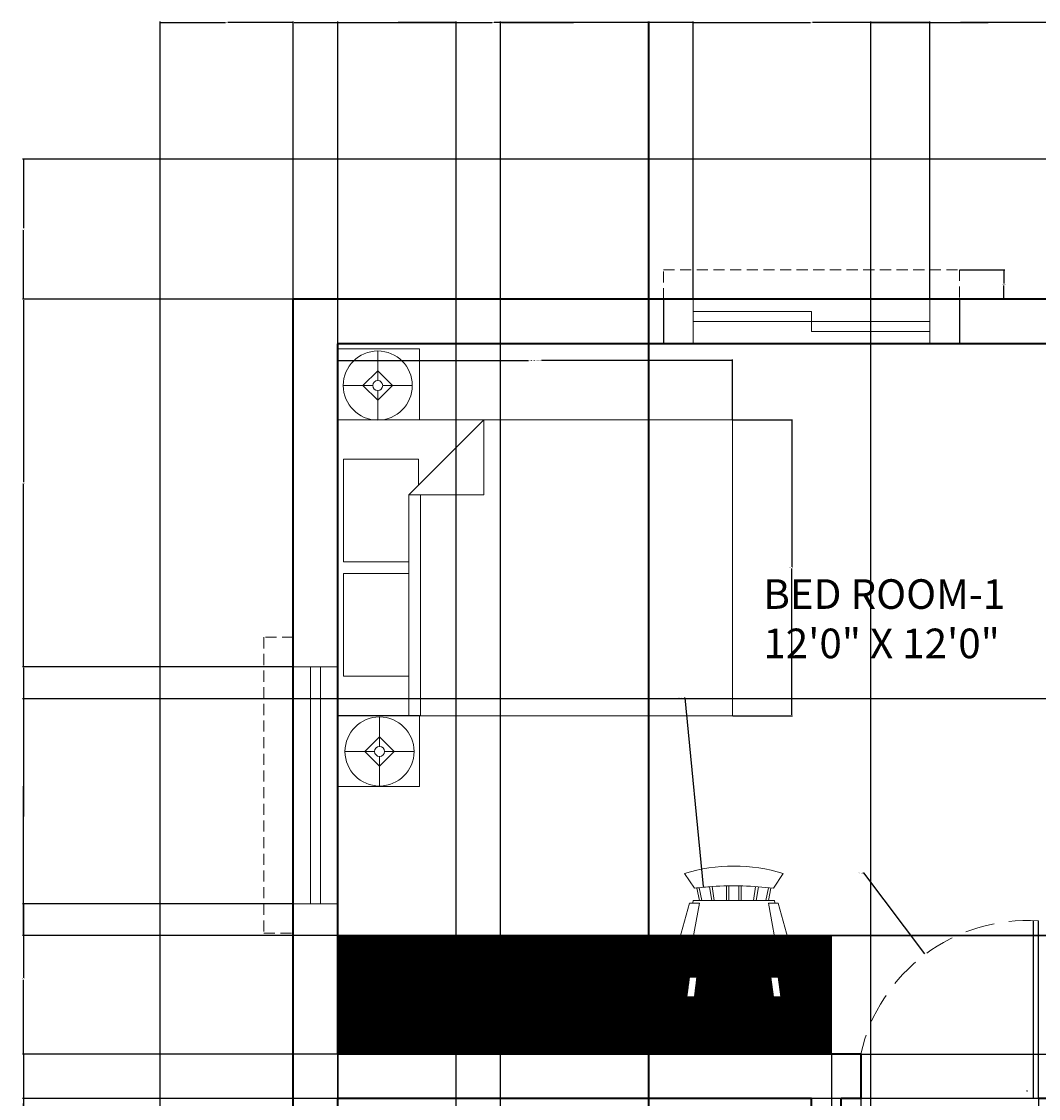
# Model space of a CAD drawing. Units: inches. Extents: x 6662 to 7211, y 5077 to 5683.
# Tile 7 of 9: x 6662 to 6868, y 5465 to 5683. Entities that reach past the tile are written whole.
import ezdxf

# ---------------------------------------------------------------- set-up
doc = ezdxf.new("R2010")
doc.units = ezdxf.units.IN
doc.header["$LTSCALE"] = 3
doc.header["$MEASUREMENT"] = 0
doc.linetypes.add('HIDDEN', pattern=[0.375, 0.25, -0.125])
for name, color, linetype, lineweight in [('A-ANNO-DIMS', 2, 'Continuous', 18), ('A-AREA-IDEN', 7, 'Continuous', 18), ('A-DOOR', 4, 'Continuous', 25), ('A-DOOR-HIDN', 4, 'HIDDEN', 13), ('A-FLOR-CASE', 8, 'Continuous', 20), ('A-FLOR-CASE-PATT', 241, 'Continuous', 13), ('A-FURN', 8, 'Continuous', 18), ('A-GLAZ', 4, 'Continuous', 18), ('A-GLAZ-OVHD', 4, 'HIDDEN', 13), ('A-WALL', 7, 'Continuous', 35)]:
    doc.layers.add(name, color=color, linetype=linetype, lineweight=lineweight)
doc.styles.get("Standard").update_dxf_attribs({"font": 'arial.ttf'})
doc.dimstyles.get("Standard").update_dxf_attribs({"dimtxt": 0.18, "dimasz": 0.18, "dimexe": 0.18, "dimexo": 0.0625, "dimgap": 0.09, "dimtad": 0, "dimtih": 1, "dimtoh": 1, "dimdec": 4, "dimzin": 0, "dimdsep": 46, "dimtxsty": 'Standard', "dimcen": 0.09, "dimadec": 0, "dimazin": 0, "dimtfac": 1, "dimtdec": 4, "dimtofl": 0, "dimtmove": 0, "dimatfit": 3, "dimfxl": 1, "dimtolj": 1, "dimtzin": 0, "dimarcsym": 0})

# ---------------------------------------------------------------- blocks, each defined once
blk = doc.blocks.new('Chair - Rocking')
for p, q in [((-8, -4.5), (-10, -1.5)), ((8, -4.5), (10, -1.5)), ((-4.5, -7), (-4.96674, -4.19951)), ((-4, -7), (-4.40532, -4.16272)), ((-1.5, -4.05012), (-1.5, -7)), ((-1, -7), (-1, -4.05012)), ((1, -7), (1, -4.04655)), ((1.5, -4.05012), (1.5, -7)), ((4, -7), (4.40187, -4.18694)), ((4.5, -7), (4.96761, -4.19437)), ((-7.5, -4.5), (-7, -7)), ((-6.5, -7), (-7.02225, -4.43)), ((6.5, -7), (7, -4.4057)), ((7.5, -4.5), (7, -7)), ((-9, -7.5), (-12, -18.49999)), ((-7, -7.5), (-9, -7.5)), ((-9, -18.49999), (-7, -7.5)), ((-8.23428, -6.99939), (-8.3093, -7.47958)), ((-8.23041, -7), (8.23915, -7)), ((7, -7.5), (9, -7.5)), ((9, -18.49999), (7, -7.5)), ((8.31071, -7.48854), (8.23449, -7.00073)), ((9, -7.5), (12, -18.49999)), ((-10.36644, -20.64523), (-10.5, -21.49999)), ((10.5, -21.49999), (10.3575, -20.58798)), ((-9, -22.49999), (-9.5, -26.49999)), ((0, -22.49999), (-9.5, -22.49999)), ((-8, -26.49999), (-7.5, -22.49999)), ((0, -22.49999), (9.5, -22.49999)), ((8, -26.49999), (7.5, -22.49999)), ((9, -22.49999), (9.5, -26.49999)), ((-9.5, -26.49999), (-8, -26.49999)), ((9.5, -26.49999), (8, -26.49999))]:
    blk.add_line(p, q)
for centre, radius, start, end in [((0, -34.08333), 34.08333, 72.93847, 107.0615), ((0, -68.25004), 64.25, 93.92211, 97.15267), ((0, -68.25004), 64.25, 82.84733, 93.92211), ((-10.5, -18.99999), 1.58114, 161.5651, 18.43495), ((10.5, -18.99999), 1.58114, 161.5651, 18.43495), ((-9.5, -21.49999), 1, 180, 270), ((9.5, -21.49999), 1, 270, 0)]:
    blk.add_arc(centre, radius, start, end)
blk = doc.blocks.new('Bed - Queen')
for p, q in [((0, -80.00003), (0, 0)), ((0, 0), (59.99999, 0)), ((59.99999, 0), (59.99999, -80.00003)), ((7.99999, -1.2), (28.79998, -1.2)), ((7.99999, -14.4), (7.99999, -1.2)), ((28.79998, -1.2), (28.79998, -14.4)), ((31.19999, -1.2), (51.99999, -1.2)), ((31.19999, -14.4), (31.19999, -1.2)), ((51.99999, -1.2), (51.99999, -16.4)), ((0, -14.4), (44.8, -14.4)), ((59.99999, -29.6), (44.8, -14.4)), ((44.8, -14.4), (44.8, -29.6)), ((44.8, -16.8), (0, -16.8)), ((51.99999, -16.4), (46.79936, -16.4)), ((44.8, -29.6), (59.99999, -29.6)), ((59.99999, -80.00003), (0, -80.00003))]:
    blk.add_line(p, q)
blk = doc.blocks.new('Lamp - Table')
for p, q in [((0, 7), (0, 1)), ((0, 3), (-3, 0)), ((3, 0), (0, 3)), ((-1, 0), (-7, 0)), ((-3, 0), (0, -3)), ((0, -3), (3, 0)), ((1, 0), (7, 0)), ((0, -1), (0, -7))]:
    blk.add_line(p, q)
for radius in [7, 1]:
    blk.add_circle((0, 0), radius)
blk = doc.blocks.new('WIN-SLIDER-48IN')
for p, q in [((0, 0), (0, 9)), ((48, 0), (48, 9)), ((0, 6.5), (24, 6.5)), ((0, 4.5), (48, 4.5)), ((24, 2.5), (24, 6.5)), ((24, 2.5), (48, 2.5))]:
    blk.add_line(p, q)
blk = doc.blocks.new('WIN-HOOD-48IN')
at = {"ltscale": 3}
for p, q in [((0, 0), (0, 6)), ((0, 6), (54, 6)), ((54, 6), (60, 6)), ((60, 6), (60, 0)), ((6, 0), (0, 0))]:
    blk.add_line(p, q, dxfattribs=at)
blk = doc.blocks.new('BEDSIDE-TABLE')
blk.add_lwpolyline([(0, 14.35), (16.56, 14.35), (16.56, 0), (0, 0)], close=True)
blk = doc.blocks.new('*D14')
at = {"layer": 'A-ANNO-DIMS', "color": 0, "lineweight": -2, "ltscale": 3, "transparency": 16777216}
for p, q in [((6725.86, 5602.25), (6725.86, 5614.37)), ((6726.04, 5614.19), (6764.55, 5614.19)), ((6805.68, 5614.19), (6767.16, 5614.19)), ((6805.86, 5602.25), (6805.86, 5614.37))]:
    blk.add_line(p, q, dxfattribs=at)
at = {"layer": 'A-ANNO-DIMS', "color": 0, "ltscale": 3, "transparency": 16777216}
for points in [[(6726.04, 5614.22), (6726.04, 5614.16), (6725.86, 5614.19)], [(6805.68, 5614.22), (6805.68, 5614.16), (6805.86, 5614.19)]]:
    blk.add_solid(points, dxfattribs=at)
at = {"layer": 'Defpoints', "color": 0, "ltscale": 3, "transparency": 16777216}
for p in [(6725.86, 5614.19), (6725.86, 5602.19), (6805.86, 5602.19)]:
    blk.add_point(p, dxfattribs=at)
at = {"layer": 'A-ANNO-DIMS', "color": 0, "ltscale": 3, "transparency": 16777216, "insert": (6765.86, 5614.19), "char_height": 0.18, "attachment_point": 5}
blk.add_mtext('\\A1;QUEEN BED 80 TYP.', dxfattribs=at)
blk = doc.blocks.new('*D15')
at = {"layer": 'A-ANNO-DIMS', "color": 0, "lineweight": -2, "ltscale": 3, "transparency": 16777216}
for p, q in [((6805.92, 5602.19), (6818.04, 5602.19)), ((6817.86, 5602.01), (6817.86, 5572.37)), ((6817.86, 5542.37), (6817.86, 5572.01)), ((6805.92, 5542.19), (6818.04, 5542.19))]:
    blk.add_line(p, q, dxfattribs=at)
at = {"layer": 'A-ANNO-DIMS', "color": 0, "ltscale": 3, "transparency": 16777216}
for points in [[(6817.83, 5602.01), (6817.89, 5602.01), (6817.86, 5602.19)], [(6817.83, 5542.37), (6817.89, 5542.37), (6817.86, 5542.19)]]:
    blk.add_solid(points, dxfattribs=at)
at = {"layer": 'Defpoints', "color": 0, "ltscale": 3, "transparency": 16777216}
for p in [(6805.86, 5602.19), (6817.86, 5602.19), (6805.86, 5542.19)]:
    blk.add_point(p, dxfattribs=at)
at = {"layer": 'A-ANNO-DIMS', "color": 0, "ltscale": 3, "transparency": 16777216, "insert": (6817.86, 5572.19), "char_height": 0.18, "attachment_point": 5}
blk.add_mtext('\\A1;60 TYP.', dxfattribs=at)
blk = doc.blocks.new('*D22')
at = {"layer": 'A-ANNO-DIMS', "color": 0, "lineweight": -2, "ltscale": 3, "transparency": 16777216}
for p, q in [((6791.86, 5626.54), (6791.86, 5617.42)), ((6851.86, 5626.54), (6851.86, 5617.42)), ((6792.04, 5617.6), (6820.33, 5617.6)), ((6851.68, 5617.6), (6823.39, 5617.6))]:
    blk.add_line(p, q, dxfattribs=at)
at = {"layer": 'A-ANNO-DIMS', "color": 0, "ltscale": 3, "transparency": 16777216}
for points in [[(6792.04, 5617.63), (6792.04, 5617.57), (6791.86, 5617.6)], [(6851.68, 5617.63), (6851.68, 5617.57), (6851.86, 5617.6)]]:
    blk.add_solid(points, dxfattribs=at)
at = {"layer": 'Defpoints', "color": 0, "ltscale": 3, "transparency": 16777216}
for p in [(6791.86, 5626.6), (6851.86, 5626.6), (6851.86, 5617.6)]:
    blk.add_point(p, dxfattribs=at)
at = {"layer": 'A-ANNO-DIMS', "color": 0, "ltscale": 3, "transparency": 16777216, "insert": (6821.86, 5617.6), "char_height": 0.18, "attachment_point": 5}
blk.add_mtext('\\A1;WINDOW HOOD 60 TYP.', dxfattribs=at)
blk = doc.blocks.new('*D23')
at = {"layer": 'A-ANNO-DIMS', "color": 0, "lineweight": -2, "ltscale": 3, "transparency": 16777216}
for p, q in [((6851.92, 5632.6), (6861.04, 5632.6)), ((6860.86, 5632.42), (6860.86, 5629.78)), ((6860.86, 5626.78), (6860.86, 5629.42)), ((6851.92, 5626.6), (6861.04, 5626.6))]:
    blk.add_line(p, q, dxfattribs=at)
at = {"layer": 'A-ANNO-DIMS', "color": 0, "ltscale": 3, "transparency": 16777216}
for points in [[(6860.83, 5632.42), (6860.89, 5632.42), (6860.86, 5632.6)], [(6860.83, 5626.78), (6860.89, 5626.78), (6860.86, 5626.6)]]:
    blk.add_solid(points, dxfattribs=at)
at = {"layer": 'Defpoints', "color": 0, "ltscale": 3, "transparency": 16777216}
for p in [(6851.86, 5632.6), (6860.86, 5632.6), (6851.86, 5626.6)]:
    blk.add_point(p, dxfattribs=at)
at = {"layer": 'A-ANNO-DIMS', "color": 0, "ltscale": 3, "transparency": 16777216, "insert": (6860.86, 5629.6), "char_height": 0.18, "attachment_point": 5}
blk.add_mtext('\\A1;6 TYP.', dxfattribs=at)
blk = doc.blocks.new('*D42')
at = {"layer": 'A-ANNO-DIMS', "color": 0, "lineweight": -2, "ltscale": 3, "transparency": 16777216}
for p, q in [((6689.86, 5392.66), (6689.86, 5682.9)), ((6690.04, 5682.72), (6703.14, 5682.72)), ((6716.68, 5682.72), (6703.58, 5682.72)), ((6716.86, 5626.66), (6716.86, 5682.9))]:
    blk.add_line(p, q, dxfattribs=at)
at = {"layer": 'A-ANNO-DIMS', "color": 0, "ltscale": 3, "transparency": 16777216}
for points in [[(6690.04, 5682.75), (6690.04, 5682.69), (6689.86, 5682.72)], [(6716.68, 5682.75), (6716.68, 5682.69), (6716.86, 5682.72)]]:
    blk.add_solid(points, dxfattribs=at)
at = {"layer": 'Defpoints', "color": 0, "ltscale": 3, "transparency": 16777216}
for p in [(6716.86, 5682.72), (6716.86, 5626.6), (6689.86, 5392.6)]:
    blk.add_point(p, dxfattribs=at)
at = {"layer": 'A-ANNO-DIMS', "color": 0, "ltscale": 3, "transparency": 16777216, "insert": (6703.36, 5682.72), "char_height": 0.18, "attachment_point": 5}
blk.add_mtext('\\A1;27', dxfattribs=at)
blk = doc.blocks.new('*D43')
at = {"layer": 'A-ANNO-DIMS', "color": 0, "lineweight": -2, "ltscale": 3, "transparency": 16777216}
for p, q in [((6716.86, 5626.66), (6716.86, 5682.9)), ((6717.04, 5682.72), (6757.16, 5682.72)), ((6797.68, 5682.72), (6757.56, 5682.72)), ((6797.86, 5626.66), (6797.86, 5682.9))]:
    blk.add_line(p, q, dxfattribs=at)
at = {"layer": 'A-ANNO-DIMS', "color": 0, "ltscale": 3, "transparency": 16777216}
for points in [[(6717.04, 5682.75), (6717.04, 5682.69), (6716.86, 5682.72)], [(6797.68, 5682.75), (6797.68, 5682.69), (6797.86, 5682.72)]]:
    blk.add_solid(points, dxfattribs=at)
at = {"layer": 'Defpoints', "color": 0, "ltscale": 3, "transparency": 16777216}
for p in [(6797.86, 5682.72), (6716.86, 5626.6), (6797.86, 5626.6)]:
    blk.add_point(p, dxfattribs=at)
at = {"layer": 'A-ANNO-DIMS', "color": 0, "ltscale": 3, "transparency": 16777216, "insert": (6757.36, 5682.72), "char_height": 0.18, "attachment_point": 5}
blk.add_mtext('\\A1;81', dxfattribs=at)
blk = doc.blocks.new('*D44')
at = {"layer": 'A-ANNO-DIMS', "color": 0, "lineweight": -2, "ltscale": 3, "transparency": 16777216}
for p, q in [((6797.86, 5626.66), (6797.86, 5682.9)), ((6798.04, 5682.72), (6821.64, 5682.72)), ((6845.68, 5682.72), (6822.08, 5682.72)), ((6845.86, 5626.66), (6845.86, 5682.9))]:
    blk.add_line(p, q, dxfattribs=at)
at = {"layer": 'A-ANNO-DIMS', "color": 0, "ltscale": 3, "transparency": 16777216}
for points in [[(6798.04, 5682.75), (6798.04, 5682.69), (6797.86, 5682.72)], [(6845.68, 5682.75), (6845.68, 5682.69), (6845.86, 5682.72)]]:
    blk.add_solid(points, dxfattribs=at)
at = {"layer": 'Defpoints', "color": 0, "ltscale": 3, "transparency": 16777216}
for p in [(6845.86, 5682.72), (6797.86, 5626.6), (6845.86, 5626.6)]:
    blk.add_point(p, dxfattribs=at)
at = {"layer": 'A-ANNO-DIMS', "color": 0, "ltscale": 3, "transparency": 16777216, "insert": (6821.86, 5682.72), "char_height": 0.18, "attachment_point": 5}
blk.add_mtext('\\A1;48', dxfattribs=at)
blk = doc.blocks.new('*D45')
at = {"layer": 'A-ANNO-DIMS', "color": 0, "lineweight": -2, "ltscale": 3, "transparency": 16777216}
for p, q in [((6845.86, 5626.66), (6845.86, 5682.9)), ((6846.04, 5682.72), (6857.64, 5682.72)), ((6869.68, 5682.72), (6858.08, 5682.72)), ((6869.86, 5655.08), (6869.86, 5682.9))]:
    blk.add_line(p, q, dxfattribs=at)
at = {"layer": 'A-ANNO-DIMS', "color": 0, "ltscale": 3, "transparency": 16777216}
for points in [[(6846.04, 5682.75), (6846.04, 5682.69), (6845.86, 5682.72)], [(6869.68, 5682.75), (6869.68, 5682.69), (6869.86, 5682.72)]]:
    blk.add_solid(points, dxfattribs=at)
at = {"layer": 'Defpoints', "color": 0, "ltscale": 3, "transparency": 16777216}
for p in [(6869.86, 5682.72), (6869.86, 5655.02), (6845.86, 5626.6)]:
    blk.add_point(p, dxfattribs=at)
at = {"layer": 'A-ANNO-DIMS', "color": 0, "ltscale": 3, "transparency": 16777216, "insert": (6857.86, 5682.72), "char_height": 0.18, "attachment_point": 5}
blk.add_mtext('\\A1;24', dxfattribs=at)
blk = doc.blocks.new('*D50')
at = {"layer": 'A-ANNO-DIMS', "color": 0, "lineweight": -2, "ltscale": 3, "transparency": 16777216}
for p, q in [((6869.8, 5655.02), (6661.98, 5655.02)), ((6662.16, 5654.84), (6662.16, 5640.99)), ((6662.16, 5626.78), (6662.16, 5640.63)), ((6716.8, 5626.6), (6661.98, 5626.6))]:
    blk.add_line(p, q, dxfattribs=at)
at = {"layer": 'A-ANNO-DIMS', "color": 0, "ltscale": 3, "transparency": 16777216}
for points in [[(6662.13, 5654.84), (6662.19, 5654.84), (6662.16, 5655.02)], [(6662.13, 5626.78), (6662.19, 5626.78), (6662.16, 5626.6)]]:
    blk.add_solid(points, dxfattribs=at)
at = {"layer": 'Defpoints', "color": 0, "ltscale": 3, "transparency": 16777216}
for p in [(6662.16, 5655.02), (6869.86, 5655.02), (6716.86, 5626.6)]:
    blk.add_point(p, dxfattribs=at)
at = {"layer": 'A-ANNO-DIMS', "color": 0, "ltscale": 3, "transparency": 16777216, "insert": (6662.16, 5640.81), "char_height": 0.18, "attachment_point": 5}
blk.add_mtext('\\A1;28.423', dxfattribs=at)
blk = doc.blocks.new('*D51')
at = {"layer": 'A-ANNO-DIMS', "color": 0, "lineweight": -2, "ltscale": 3, "transparency": 16777216}
for p, q in [((6716.8, 5626.6), (6661.98, 5626.6)), ((6662.16, 5626.42), (6662.16, 5589.52)), ((6662.16, 5552.26), (6662.16, 5589.16)), ((6716.8, 5552.08), (6661.98, 5552.08))]:
    blk.add_line(p, q, dxfattribs=at)
at = {"layer": 'A-ANNO-DIMS', "color": 0, "ltscale": 3, "transparency": 16777216}
for points in [[(6662.13, 5626.42), (6662.19, 5626.42), (6662.16, 5626.6)], [(6662.13, 5552.26), (6662.19, 5552.26), (6662.16, 5552.08)]]:
    blk.add_solid(points, dxfattribs=at)
at = {"layer": 'Defpoints', "color": 0, "ltscale": 3, "transparency": 16777216}
for p in [(6716.86, 5626.6), (6662.16, 5552.08), (6716.86, 5552.08)]:
    blk.add_point(p, dxfattribs=at)
at = {"layer": 'A-ANNO-DIMS', "color": 0, "ltscale": 3, "transparency": 16777216, "insert": (6662.16, 5589.34), "char_height": 0.18, "attachment_point": 5}
blk.add_mtext('\\A1;74.52', dxfattribs=at)
blk = doc.blocks.new('*D52')
at = {"layer": 'A-ANNO-DIMS', "color": 0, "lineweight": -2, "ltscale": 3, "transparency": 16777216}
for p, q in [((6716.8, 5552.08), (6661.98, 5552.08)), ((6662.16, 5551.9), (6662.16, 5528.26)), ((6662.16, 5504.26), (6662.16, 5527.9)), ((6716.8, 5504.08), (6661.98, 5504.08))]:
    blk.add_line(p, q, dxfattribs=at)
at = {"layer": 'A-ANNO-DIMS', "color": 0, "ltscale": 3, "transparency": 16777216}
for points in [[(6662.13, 5551.9), (6662.19, 5551.9), (6662.16, 5552.08)], [(6662.13, 5504.26), (6662.19, 5504.26), (6662.16, 5504.08)]]:
    blk.add_solid(points, dxfattribs=at)
at = {"layer": 'Defpoints', "color": 0, "ltscale": 3, "transparency": 16777216}
for p in [(6716.86, 5552.08), (6662.16, 5504.08), (6716.86, 5504.08)]:
    blk.add_point(p, dxfattribs=at)
at = {"layer": 'A-ANNO-DIMS', "color": 0, "ltscale": 3, "transparency": 16777216, "insert": (6662.16, 5528.08), "char_height": 0.18, "attachment_point": 5}
blk.add_mtext('\\A1;48', dxfattribs=at)
blk = doc.blocks.new('*D53')
at = {"layer": 'A-ANNO-DIMS', "color": 0, "lineweight": -2, "ltscale": 3, "transparency": 16777216}
for p, q in [((6716.8, 5504.08), (6661.98, 5504.08)), ((6662.16, 5503.9), (6662.16, 5489.02)), ((6662.16, 5473.78), (6662.16, 5488.66)), ((6725.8, 5473.6), (6661.98, 5473.6))]:
    blk.add_line(p, q, dxfattribs=at)
at = {"layer": 'A-ANNO-DIMS', "color": 0, "ltscale": 3, "transparency": 16777216}
for points in [[(6662.13, 5503.9), (6662.19, 5503.9), (6662.16, 5504.08)], [(6662.13, 5473.78), (6662.19, 5473.78), (6662.16, 5473.6)]]:
    blk.add_solid(points, dxfattribs=at)
at = {"layer": 'Defpoints', "color": 0, "ltscale": 3, "transparency": 16777216}
for p in [(6716.86, 5504.08), (6662.16, 5473.6), (6725.86, 5473.6)]:
    blk.add_point(p, dxfattribs=at)
at = {"layer": 'A-ANNO-DIMS', "color": 0, "ltscale": 3, "transparency": 16777216, "insert": (6662.16, 5488.84), "char_height": 0.18, "attachment_point": 5}
blk.add_mtext('\\A1;30.48', dxfattribs=at)
blk = doc.blocks.new('*D54')
at = {"layer": 'A-ANNO-DIMS', "color": 0, "lineweight": -2, "ltscale": 3, "transparency": 16777216}
for p, q in [((6725.8, 5473.6), (6661.98, 5473.6)), ((6662.16, 5473.42), (6662.16, 5463.93)), ((6662.16, 5454.09), (6662.16, 5463.57)), ((6716.8, 5453.91), (6661.98, 5453.91))]:
    blk.add_line(p, q, dxfattribs=at)
at = {"layer": 'A-ANNO-DIMS', "color": 0, "ltscale": 3, "transparency": 16777216}
for points in [[(6662.13, 5473.42), (6662.19, 5473.42), (6662.16, 5473.6)], [(6662.13, 5454.09), (6662.19, 5454.09), (6662.16, 5453.91)]]:
    blk.add_solid(points, dxfattribs=at)
at = {"layer": 'Defpoints', "color": 0, "ltscale": 3, "transparency": 16777216}
for p in [(6662.16, 5473.6), (6725.86, 5473.6), (6716.86, 5453.91)]:
    blk.add_point(p, dxfattribs=at)
at = {"layer": 'A-ANNO-DIMS', "color": 0, "ltscale": 3, "transparency": 16777216, "insert": (6662.16, 5463.75), "char_height": 0.18, "attachment_point": 5}
blk.add_mtext('\\A1;19.69', dxfattribs=at)
blk = doc.blocks.new('*D63')
at = {"layer": 'A-ANNO-DIMS', "color": 0, "lineweight": -2, "ltscale": 3, "transparency": 16777216}
for p, q in [((6758.86, 5332.16), (6758.86, 5682.9)), ((6759.04, 5682.72), (6773.64, 5682.72)), ((6788.68, 5682.72), (6774.08, 5682.72)), ((6788.86, 5332.16), (6788.86, 5682.9))]:
    blk.add_line(p, q, dxfattribs=at)
at = {"layer": 'A-ANNO-DIMS', "color": 0, "ltscale": 3, "transparency": 16777216}
for points in [[(6759.04, 5682.75), (6759.04, 5682.69), (6758.86, 5682.72)], [(6788.68, 5682.75), (6788.68, 5682.69), (6788.86, 5682.72)]]:
    blk.add_solid(points, dxfattribs=at)
at = {"layer": 'Defpoints', "color": 0, "ltscale": 3, "transparency": 16777216}
for p in [(6788.86, 5682.72), (6758.86, 5332.1), (6788.86, 5332.1)]:
    blk.add_point(p, dxfattribs=at)
at = {"layer": 'A-ANNO-DIMS', "color": 0, "ltscale": 3, "transparency": 16777216, "insert": (6773.86, 5682.72), "char_height": 0.18, "attachment_point": 5}
blk.add_mtext('\\A1;30', dxfattribs=at)
blk = doc.blocks.new('*D64')
at = {"layer": 'A-ANNO-DIMS', "color": 0, "lineweight": -2, "ltscale": 3, "transparency": 16777216}
for p, q in [((6833.86, 5332.16), (6833.86, 5682.9)), ((6834.04, 5682.72), (6851.64, 5682.72)), ((6869.68, 5682.72), (6852.08, 5682.72)), ((6869.86, 5332.16), (6869.86, 5682.9))]:
    blk.add_line(p, q, dxfattribs=at)
at = {"layer": 'A-ANNO-DIMS', "color": 0, "ltscale": 3, "transparency": 16777216}
for points in [[(6834.04, 5682.75), (6834.04, 5682.69), (6833.86, 5682.72)], [(6869.68, 5682.75), (6869.68, 5682.69), (6869.86, 5682.72)]]:
    blk.add_solid(points, dxfattribs=at)
at = {"layer": 'Defpoints', "color": 0, "ltscale": 3, "transparency": 16777216}
for p in [(6869.86, 5682.72), (6833.86, 5332.1), (6869.86, 5332.1)]:
    blk.add_point(p, dxfattribs=at)
at = {"layer": 'A-ANNO-DIMS', "color": 0, "ltscale": 3, "transparency": 16777216, "insert": (6851.86, 5682.72), "char_height": 0.18, "attachment_point": 5}
blk.add_mtext('\\A1;36', dxfattribs=at)
blk = doc.blocks.new('*D65')
at = {"layer": 'A-ANNO-DIMS', "color": 0, "lineweight": -2, "ltscale": 3, "transparency": 16777216}
for p, q in [((6831.86, 5464.54), (6831.86, 5076.72)), ((6867.86, 5464.54), (6867.86, 5076.72)), ((6832.04, 5076.9), (6849.64, 5076.9)), ((6867.68, 5076.9), (6850.08, 5076.9))]:
    blk.add_line(p, q, dxfattribs=at)
at = {"layer": 'A-ANNO-DIMS', "color": 0, "ltscale": 3, "transparency": 16777216}
for points in [[(6832.04, 5076.93), (6832.04, 5076.87), (6831.86, 5076.9)], [(6867.68, 5076.93), (6867.68, 5076.87), (6867.86, 5076.9)]]:
    blk.add_solid(points, dxfattribs=at)
at = {"layer": 'Defpoints', "color": 0, "ltscale": 3, "transparency": 16777216}
for p in [(6831.86, 5464.6), (6867.86, 5464.6), (6867.86, 5076.9)]:
    blk.add_point(p, dxfattribs=at)
at = {"layer": 'A-ANNO-DIMS', "color": 0, "ltscale": 3, "transparency": 16777216, "insert": (6849.86, 5076.9), "char_height": 0.18, "attachment_point": 5}
blk.add_mtext('\\A1;36', dxfattribs=at)
blk = doc.blocks.new('*D73')
at = {"layer": 'A-ANNO-DIMS', "color": 0, "lineweight": -2, "ltscale": 3, "transparency": 16777216}
for p, q in [((6725.86, 5179.16), (6725.86, 5682.9)), ((6726.04, 5682.72), (6757.03, 5682.72)), ((6788.79, 5682.72), (6757.79, 5682.72)), ((6788.97, 5179.16), (6788.97, 5682.9))]:
    blk.add_line(p, q, dxfattribs=at)
at = {"layer": 'A-ANNO-DIMS', "color": 0, "ltscale": 3, "transparency": 16777216}
for points in [[(6726.04, 5682.75), (6726.04, 5682.69), (6725.86, 5682.72)], [(6788.79, 5682.75), (6788.79, 5682.69), (6788.97, 5682.72)]]:
    blk.add_solid(points, dxfattribs=at)
at = {"layer": 'Defpoints', "color": 0, "ltscale": 3, "transparency": 16777216}
for p in [(6788.97, 5682.72), (6725.86, 5179.1), (6788.97, 5179.1)]:
    blk.add_point(p, dxfattribs=at)
at = {"layer": 'A-ANNO-DIMS', "color": 0, "ltscale": 3, "transparency": 16777216, "insert": (6757.41, 5682.72), "char_height": 0.18, "attachment_point": 5}
blk.add_mtext('\\A1;63.11', dxfattribs=at)
blk = doc.blocks.new('*D76')
at = {"layer": 'A-ANNO-DIMS', "color": 0, "lineweight": -2, "ltscale": 3, "transparency": 16777216}
for p, q in [((7167.8, 5464.6), (6661.98, 5464.6)), ((6662.16, 5464.42), (6662.16, 5449.65)), ((6662.16, 5434.53), (6662.16, 5449.29)), ((7167.8, 5434.35), (6661.98, 5434.35))]:
    blk.add_line(p, q, dxfattribs=at)
at = {"layer": 'A-ANNO-DIMS', "color": 0, "ltscale": 3, "transparency": 16777216}
for points in [[(6662.13, 5464.42), (6662.19, 5464.42), (6662.16, 5464.6)], [(6662.13, 5434.53), (6662.19, 5434.53), (6662.16, 5434.35)]]:
    blk.add_solid(points, dxfattribs=at)
at = {"layer": 'Defpoints', "color": 0, "ltscale": 3, "transparency": 16777216}
for p in [(7167.86, 5464.6), (6662.16, 5434.35), (7167.86, 5434.35)]:
    blk.add_point(p, dxfattribs=at)
at = {"layer": 'A-ANNO-DIMS', "color": 0, "ltscale": 3, "transparency": 16777216, "insert": (6662.16, 5449.47), "char_height": 0.18, "attachment_point": 5}
blk.add_mtext('\\A1;30.25', dxfattribs=at)
blk = doc.blocks.new('*D79')
at = {"layer": 'A-ANNO-DIMS', "color": 0, "lineweight": -2, "ltscale": 3, "transparency": 16777216}
for p, q in [((6725.86, 5473.54), (6725.86, 5076.72)), ((6825.9, 5473.54), (6825.9, 5076.72)), ((6726.04, 5076.9), (6775.42, 5076.9)), ((6825.72, 5076.9), (6776.33, 5076.9))]:
    blk.add_line(p, q, dxfattribs=at)
at = {"layer": 'A-ANNO-DIMS', "color": 0, "ltscale": 3, "transparency": 16777216}
for points in [[(6726.04, 5076.93), (6726.04, 5076.87), (6725.86, 5076.9)], [(6825.72, 5076.93), (6825.72, 5076.87), (6825.9, 5076.9)]]:
    blk.add_solid(points, dxfattribs=at)
at = {"layer": 'Defpoints', "color": 0, "ltscale": 3, "transparency": 16777216}
for p in [(6725.86, 5473.6), (6825.9, 5473.6), (6825.9, 5076.9)]:
    blk.add_point(p, dxfattribs=at)
at = {"layer": 'A-ANNO-DIMS', "color": 0, "ltscale": 3, "transparency": 16777216, "insert": (6775.88, 5076.9), "char_height": 0.18, "attachment_point": 5}
blk.add_mtext('\\A1;100.04', dxfattribs=at)
blk = doc.blocks.new('*D80')
at = {"layer": 'A-ANNO-DIMS', "color": 0, "lineweight": -2, "ltscale": 3, "transparency": 16777216}
for p, q in [((6825.96, 5497.6), (7210.74, 5497.6)), ((7210.56, 5497.42), (7210.56, 5485.78)), ((7210.56, 5473.78), (7210.56, 5485.42)), ((6825.96, 5473.6), (7210.74, 5473.6))]:
    blk.add_line(p, q, dxfattribs=at)
at = {"layer": 'A-ANNO-DIMS', "color": 0, "ltscale": 3, "transparency": 16777216}
for points in [[(7210.53, 5497.42), (7210.59, 5497.42), (7210.56, 5497.6)], [(7210.53, 5473.78), (7210.59, 5473.78), (7210.56, 5473.6)]]:
    blk.add_solid(points, dxfattribs=at)
at = {"layer": 'Defpoints', "color": 0, "ltscale": 3, "transparency": 16777216}
for p in [(6825.9, 5497.6), (7210.56, 5497.6), (6825.9, 5473.6)]:
    blk.add_point(p, dxfattribs=at)
at = {"layer": 'A-ANNO-DIMS', "color": 0, "ltscale": 3, "transparency": 16777216, "insert": (7210.56, 5485.6), "char_height": 0.18, "attachment_point": 5}
blk.add_mtext('\\A1;24', dxfattribs=at)
blk = doc.blocks.new('*D82')
at = {"layer": 'A-ANNO-DIMS', "color": 0, "lineweight": -2, "ltscale": 3, "transparency": 16777216}
for p, q in [((7167.8, 5545.6), (6661.98, 5545.6)), ((6662.16, 5545.42), (6662.16, 5521.78)), ((6662.16, 5497.78), (6662.16, 5521.42)), ((7167.8, 5497.6), (6661.98, 5497.6))]:
    blk.add_line(p, q, dxfattribs=at)
at = {"layer": 'A-ANNO-DIMS', "color": 0, "ltscale": 3, "transparency": 16777216}
for points in [[(6662.13, 5545.42), (6662.19, 5545.42), (6662.16, 5545.6)], [(6662.13, 5497.78), (6662.19, 5497.78), (6662.16, 5497.6)]]:
    blk.add_solid(points, dxfattribs=at)
at = {"layer": 'Defpoints', "color": 0, "ltscale": 3, "transparency": 16777216}
for p in [(6662.16, 5545.6), (7167.86, 5545.6), (7167.86, 5497.6)]:
    blk.add_point(p, dxfattribs=at)
at = {"layer": 'A-ANNO-DIMS', "color": 0, "ltscale": 3, "transparency": 16777216, "insert": (6662.16, 5521.6), "char_height": 0.18, "attachment_point": 5}
blk.add_mtext('\\A1;48', dxfattribs=at)
blk = doc.blocks.new('*D84')
at = {"layer": 'A-ANNO-DIMS', "color": 0, "lineweight": -2, "ltscale": 3, "transparency": 16777216}
for p, q in [((6725.86, 5388.16), (6725.86, 5682.9)), ((6726.04, 5682.72), (6737.64, 5682.72)), ((6749.68, 5682.72), (6738.08, 5682.72)), ((6749.86, 5388.16), (6749.86, 5682.9))]:
    blk.add_line(p, q, dxfattribs=at)
at = {"layer": 'A-ANNO-DIMS', "color": 0, "ltscale": 3, "transparency": 16777216}
for points in [[(6726.04, 5682.75), (6726.04, 5682.69), (6725.86, 5682.72)], [(6749.68, 5682.75), (6749.68, 5682.69), (6749.86, 5682.72)]]:
    blk.add_solid(points, dxfattribs=at)
at = {"layer": 'Defpoints', "color": 0, "ltscale": 3, "transparency": 16777216}
for p in [(6725.86, 5682.72), (6725.86, 5388.1), (6749.86, 5388.1)]:
    blk.add_point(p, dxfattribs=at)
at = {"layer": 'A-ANNO-DIMS', "color": 0, "ltscale": 3, "transparency": 16777216, "insert": (6737.86, 5682.72), "char_height": 0.18, "attachment_point": 5}
blk.add_mtext('\\A1;24', dxfattribs=at)
blk = doc.blocks.new('*D90')
at = {"layer": 'A-ANNO-DIMS', "color": 0, "lineweight": -2, "ltscale": 3, "transparency": 16777216}
for p, q in [((6832.25, 5510.34), (6832.43, 5510.34)), ((6832.43, 5510.34), (6844.75, 5493.91)), ((6865.48, 5466.15), (6865.66, 5466.15)), ((6865.57, 5466.06), (6865.57, 5466.24))]:
    blk.add_line(p, q, dxfattribs=at)
at = {"layer": 'A-ANNO-DIMS', "color": 0, "ltscale": 3, "transparency": 16777216}
blk.add_solid([(6844.77, 5493.93), (6844.72, 5493.9), (6844.85, 5493.77)], dxfattribs=at)
at = {"layer": 'Defpoints', "color": 0, "ltscale": 3, "transparency": 16777216}
for p in [(6844.85, 5493.77), (6865.57, 5466.15)]:
    blk.add_point(p, dxfattribs=at)
at = {"layer": 'A-ANNO-DIMS', "color": 0, "ltscale": 3, "transparency": 16777216, "insert": (6831.77, 5510.34), "char_height": 0.18, "attachment_point": 5}
blk.add_mtext('\\A1;R34.52', dxfattribs=at)
blk = doc.blocks.new('*D102')
at = {"layer": 'A-ANNO-DIMS', "color": 0, "lineweight": -2, "ltscale": 3, "transparency": 16777216}
for p, q in [((6796.04, 5545.78), (6796.22, 5545.78)), ((6796.22, 5545.78), (6799.92, 5507.59)), ((6806.05, 5443.46), (6806.23, 5443.46)), ((6806.14, 5443.37), (6806.14, 5443.55))]:
    blk.add_line(p, q, dxfattribs=at)
at = {"layer": 'A-ANNO-DIMS', "color": 0, "ltscale": 3, "transparency": 16777216}
blk.add_solid([(6799.95, 5507.59), (6799.89, 5507.59), (6799.94, 5507.41)], dxfattribs=at)
at = {"layer": 'Defpoints', "color": 0, "ltscale": 3, "transparency": 16777216}
for p in [(6799.94, 5507.41), (6806.14, 5443.46)]:
    blk.add_point(p, dxfattribs=at)
at = {"layer": 'A-ANNO-DIMS', "color": 0, "ltscale": 3, "transparency": 16777216, "insert": (6795.36, 5545.78), "char_height": 0.18, "attachment_point": 5}
blk.add_mtext('\\A1;4X R64.25', dxfattribs=at)

msp = doc.modelspace()

# ---------------------------------------------------------------- hatches: boundary and pattern name
at = {"layer": 'A-FLOR-CASE-PATT'}
h = msp.add_hatch(dxfattribs=at)
h.set_pattern_fill('ANSI31', color=256)
h.paths.add_polyline_path([(6869.8579, 5283.7981), (6845.8579, 5283.7981), (6845.8579, 5229.4653), (6847.018, 5229.7817, -0.54116316), (6849.0925, 5228.1371), (6849.7129, 5228.234, -0.50821327), (6851.018, 5227.2817), (6851.018, 5226.7817), (6855.018, 5227.2817), (6855.018, 5225.7817), (6851.018, 5225.2817), (6851.018, 5217.7817), (6851.018, 5210.2817), (6855.018, 5209.7817), (6855.018, 5208.2817), (6851.018, 5208.7817), (6851.018, 5208.2817, -0.41421356), (6850.018, 5207.2817), (6849.0925, 5207.4263, -0.50580924), (6847.1872, 5205.7355), (6845.8579, 5206.0981), (6845.8579, 5179.0979), (6869.8579, 5179.0979)])
h.paths.add_polyline_path([(7167.8579, 5497.5979), (7143.8579, 5497.5979), (7078.3579, 5497.5979), (7078.3579, 5473.5979), (7163.8579, 5473.5979), (7167.8579, 5473.5979)])
h.paths.add_polyline_path([(6825.9016, 5497.5979), (6725.8579, 5497.5979), (6725.8579, 5473.5979), (6825.9016, 5473.5979)])
h.paths.add_polyline_path([(6796.6359, 5485.2095), (6797.1359, 5489.2095), (6806.1359, 5489.2095), (6815.1359, 5489.2095), (6815.6359, 5485.2095), (6814.1359, 5485.2095), (6813.6359, 5489.2095), (6806.1359, 5489.2095), (6798.6359, 5489.2095), (6798.1359, 5485.2095)], flags=16)

# ---------------------------------------------------------------- linework, layer by layer
at = {"layer": 'A-DOOR'}
for p, q in [((6866.8579, 5464.5979), (6866.8579, 5500.5979)), ((6867.8579, 5464.5979), (6867.8579, 5500.5979))]:
    msp.add_line(p, q, dxfattribs=at)
at = {"layer": 'A-DOOR-HIDN', "ltscale": 8}
msp.add_arc((6865.566, 5466.1537), 34.5204, 86.193259, 167.546536, dxfattribs=at)
at = {"layer": 'A-FLOR-CASE'}
for p, q in [((6825.9016, 5497.5979), (6725.8579, 5497.5979)), ((6825.9016, 5473.5979), (6825.9016, 5497.5979))]:
    msp.add_line(p, q, dxfattribs=at)
at = {"layer": 'A-GLAZ'}
for p, q in [((6725.8579, 5552.0774), (6716.8579, 5552.0774)), ((6720.3579, 5552.0774), (6720.3579, 5504.0774)), ((6722.3579, 5552.0774), (6722.3579, 5504.0774)), ((6725.8579, 5504.0774), (6716.8579, 5504.0774))]:
    msp.add_line(p, q, dxfattribs=at)
at = {"layer": 'A-GLAZ-OVHD', "ltscale": 3}
msp.add_line((6716.8579, 5498.0774), (6716.8579, 5504.0774), dxfattribs=at)
at = {"layer": 'A-WALL'}
for p, q in [((6716.8579, 5170.0979), (6716.8579, 5626.5979)), ((7176.8579, 5626.5979), (6716.8579, 5626.5979)), ((6725.8579, 5473.5979), (6725.8579, 5617.5979)), ((6869.8579, 5617.5979), (6725.8579, 5617.5979)), ((6831.8579, 5473.5979), (6725.8579, 5473.5979)), ((6831.8579, 5473.5979), (6831.8579, 5464.5979)), ((6725.8579, 5392.5979), (6725.8579, 5464.5979)), ((6821.8579, 5464.5979), (6725.8579, 5464.5979)), ((6821.8579, 5392.5979), (6821.8579, 5464.5979)), ((6827.8579, 5332.0979), (6827.8579, 5464.5979)), ((6831.8579, 5464.5979), (6827.8579, 5464.5979)), ((6831.8579, 5464.5979), (6827.8579, 5464.5979)), ((6956.8579, 5464.5979), (6867.8579, 5464.5979))]:
    msp.add_line(p, q, dxfattribs=at)

# ---------------------------------------------------------------- block references
at = {"layer": 'A-FURN'}
for name, p in [('BEDSIDE-TABLE', (6725.858, 5602.1913)), ('Lamp - Table', (6733.9708, 5609.1173)), ('BEDSIDE-TABLE', (6725.858, 5527.8645)), ('Lamp - Table', (6734.327, 5534.9338)), ('Chair - Rocking', (6806.1359, 5511.7095))]:
    msp.add_blockref(name, p, dxfattribs=at)
at = {"layer": 'A-FURN', "rotation": 90}
msp.add_blockref('Bed - Queen', (6725.8579, 5542.191), dxfattribs=at)
at = {"layer": 'A-GLAZ'}
msp.add_blockref('WIN-SLIDER-48IN', (6797.858, 5617.598), dxfattribs=at)
at = {"layer": 'A-GLAZ-OVHD'}
msp.add_blockref('WIN-HOOD-48IN', (6791.858, 5626.598), dxfattribs=at)
at = {"layer": 'A-GLAZ-OVHD', "extrusion": (0, 0, -1), "zscale": -1, "rotation": 270}
msp.add_blockref('WIN-HOOD-48IN', (-6716.8578, 5558.0772), dxfattribs=at)

# ---------------------------------------------------------------- texts
at = {"layer": 'A-AREA-IDEN', "ltscale": 3, "insert": (6812.1068, 5569.8433), "char_height": 6, "attachment_point": 1}
msp.add_mtext_dynamic_manual_height_columns('BED ROOM-1\\P12\'0" X 12\'0"', width=381.547883, gutter_width=1, heights=[0], dxfattribs=at)

# ---------------------------------------------------------------- dimensions: what is measured, and where the dimension line sits
at = {"layer": 'A-ANNO-DIMS', "ltscale": 3}
for base, p1, p2, override, picture, middle in [((6716.8579, 5682.7209), (6689.8579, 5392.5979), (6716.8579, 5626.5979), {"dimdec": 0, "dimlfac": 1, "dimrnd": 0, "dimzin": 0, "dimdsep": 46, "dimlunit": 2}, '*D42', (6703.3579, 5682.7209)), ((6797.8579, 5682.7209), (6716.8579, 5626.5979), (6797.8579, 5626.5979), {"dimdec": 0, "dimlfac": 1, "dimrnd": 0, "dimzin": 0, "dimdsep": 46, "dimlunit": 2}, '*D43', (6757.3579, 5682.7209)), ((6788.9657, 5682.7209), (6725.8579, 5179.0979), (6788.9657, 5179.0979), {"dimdec": 2, "dimlfac": 1, "dimrnd": 0, "dimzin": 0, "dimdsep": 46, "dimlunit": 2}, '*D73', (6757.4118, 5682.7209)), ((6725.8579, 5682.7209), (6749.8579, 5388.0979), (6725.8579, 5388.0979), {"dimdec": 0, "dimlfac": 1, "dimrnd": 0, "dimzin": 0, "dimdsep": 46, "dimlunit": 2}, '*D84', (6737.8579, 5682.7209)), ((6788.8579, 5682.7209), (6758.8579, 5332.0979), (6788.8579, 5332.0979), {"dimdec": 0, "dimlfac": 1, "dimrnd": 0, "dimzin": 0, "dimdsep": 46, "dimlunit": 2}, '*D63', (6773.8579, 5682.7209)), ((6845.8579, 5682.7209), (6797.8579, 5626.5979), (6845.8579, 5626.5979), {"dimdec": 0, "dimlfac": 1, "dimrnd": 0, "dimzin": 0, "dimdsep": 46, "dimlunit": 2}, '*D44', (6821.8579, 5682.7209)), ((6869.8579, 5682.7209), (6833.8579, 5332.0979), (6869.8579, 5332.0979), {"dimdec": 0, "dimlfac": 1, "dimrnd": 0, "dimzin": 0, "dimdsep": 46, "dimlunit": 2}, '*D64', (6851.8579, 5682.7209)), ((6869.8579, 5682.7209), (6845.8579, 5626.5979), (6869.8579, 5655.0209), {"dimdec": 0, "dimlfac": 1, "dimrnd": 0, "dimzin": 0, "dimdsep": 46, "dimlunit": 2}, '*D45', (6857.8579, 5682.7209)), ((6825.9016, 5076.8979), (6725.8579, 5473.5979), (6825.9016, 5473.5979), {"dimdec": 2, "dimlfac": 1, "dimrnd": 0, "dimzin": 0, "dimdsep": 46, "dimlunit": 2}, '*D79', (6775.8797, 5076.8979)), ((6867.8579, 5076.8979), (6831.8579, 5464.5979), (6867.8579, 5464.5979), {"dimdec": 0, "dimlfac": 1, "dimrnd": 0, "dimzin": 0, "dimdsep": 46, "dimlunit": 2}, '*D65', (6849.8579, 5076.8979))]:
    dim = msp.add_linear_dim(base=base, p1=p1, p2=p2, dimstyle='Standard', override=override, dxfattribs=at)
    dim.commit()
    dim.dimension.update_dxf_attribs({"geometry": picture, "text_midpoint": middle})
for base, p1, p2, override, picture, middle in [((6662.1579, 5655.0209), (6716.8579, 5626.5979), (6869.8579, 5655.0209), {"dimdec": 3, "dimlfac": 1, "dimrnd": 0, "dimzin": 0, "dimdsep": 46, "dimlunit": 2}, '*D50', (6662.1579, 5640.8094)), ((6662.1579, 5552.0774), (6716.8579, 5626.5979), (6716.8579, 5552.0774), {"dimdec": 2, "dimlfac": 1, "dimrnd": 0, "dimzin": 0, "dimdsep": 46, "dimlunit": 2}, '*D51', (6662.1579, 5589.3376)), ((6662.1579, 5504.0774), (6716.8579, 5552.0774), (6716.8579, 5504.0774), {"dimdec": 0, "dimlfac": 1, "dimrnd": 0, "dimzin": 0, "dimdsep": 46, "dimlunit": 2}, '*D52', (6662.1579, 5528.0774)), ((6662.1579, 5545.5979), (7167.8579, 5497.5979), (7167.8579, 5545.5979), {"dimdec": 0, "dimlfac": 1, "dimrnd": 0, "dimzin": 0, "dimdsep": 46, "dimlunit": 2}, '*D82', (6662.1579, 5521.5979)), ((6662.1579, 5473.5979), (6716.8579, 5504.0774), (6725.8579, 5473.5979), {"dimdec": 2, "dimlfac": 1, "dimrnd": 0, "dimzin": 0, "dimdsep": 46, "dimlunit": 2}, '*D53', (6662.1579, 5488.8376)), ((7210.5579, 5497.5979), (6825.9016, 5473.5979), (6825.9016, 5497.5979), {"dimdec": 0, "dimlfac": 1, "dimrnd": 0, "dimzin": 0, "dimdsep": 46, "dimlunit": 2}, '*D80', (7210.5579, 5485.5979)), ((6662.1579, 5473.5979), (6716.8579, 5453.908), (6725.8579, 5473.5979), {"dimdec": 2, "dimlfac": 1, "dimrnd": 0, "dimzin": 0, "dimdsep": 46, "dimlunit": 2}, '*D54', (6662.1579, 5463.753)), ((6662.1579, 5434.3479), (7167.8579, 5464.5979), (7167.8579, 5434.3479), {"dimdec": 2, "dimlfac": 1, "dimrnd": 0, "dimzin": 0, "dimdsep": 46, "dimlunit": 2}, '*D76', (6662.1579, 5449.4729))]:
    dim = msp.add_linear_dim(base=base, p1=p1, p2=p2, angle=90, dimstyle='Standard', override=override, dxfattribs=at)
    dim.commit()
    dim.dimension.update_dxf_attribs({"geometry": picture, "text_midpoint": middle})
for base, p1, p2, angle, text, picture, middle in [((6860.8579, 5632.5979), (6851.8579, 5626.5979), (6851.8579, 5632.5979), 90, '<> TYP.', '*D23', (6860.8579, 5629.5979)), ((6725.8579, 5614.1909), (6805.8579, 5602.1909), (6725.8579, 5602.1909), 180, 'QUEEN BED <> TYP.', '*D14', (6765.8579, 5614.1909)), ((6817.8579, 5602.1909), (6805.8579, 5542.191), (6805.8579, 5602.1909), 90, '<> TYP.', '*D15', (6817.8579, 5572.1909))]:
    dim = msp.add_linear_dim(base=base, p1=p1, p2=p2, angle=angle, text=text, dimstyle='Standard', override={"dimdec": 0, "dimlfac": 1, "dimrnd": 0, "dimzin": 0, "dimdsep": 46, "dimlunit": 2}, dxfattribs=at)
    dim.commit()
    dim.dimension.update_dxf_attribs({"geometry": picture, "text_midpoint": middle})
dim = msp.add_linear_dim(base=(6851.8579, 5617.5979), p1=(6791.8579, 5626.5979), p2=(6851.8579, 5626.5979), text='WINDOW HOOD <> TYP.', dimstyle='Standard', override={"dimdec": 0, "dimlfac": 1, "dimrnd": 0, "dimzin": 0, "dimdsep": 46, "dimlunit": 2}, dxfattribs=at)
dim.commit()
dim.dimension.update_dxf_attribs({"geometry": '*D22', "text_midpoint": (6821.8579, 5617.5979)})
dim = msp.add_radius_dim(center=(6806.1359, 5443.4595), mpoint=(6799.936, 5507.4097), text='4X <>', dimstyle='Standard', override={"dimdec": 2, "dimlfac": 1, "dimrnd": 0, "dimzin": 0, "dimdsep": 46, "dimlunit": 2}, dxfattribs=at)
dim.commit()
dim.dimension.update_dxf_attribs({"geometry": '*D102', "text_midpoint": (6795.3586, 5545.7798), "dimtype": 164})
dim = msp.add_radius_dim(center=(6865.566, 5466.1537), mpoint=(6844.8539, 5493.7701), dimstyle='Standard', override={"dimdec": 2, "dimlfac": 1, "dimrnd": 0, "dimzin": 0, "dimdsep": 46, "dimlunit": 2}, dxfattribs=at)
dim.commit()
dim.dimension.update_dxf_attribs({"geometry": '*D90', "text_midpoint": (6831.7677, 5510.3399), "dimtype": 164})

doc.saveas('drawing.dxf')
